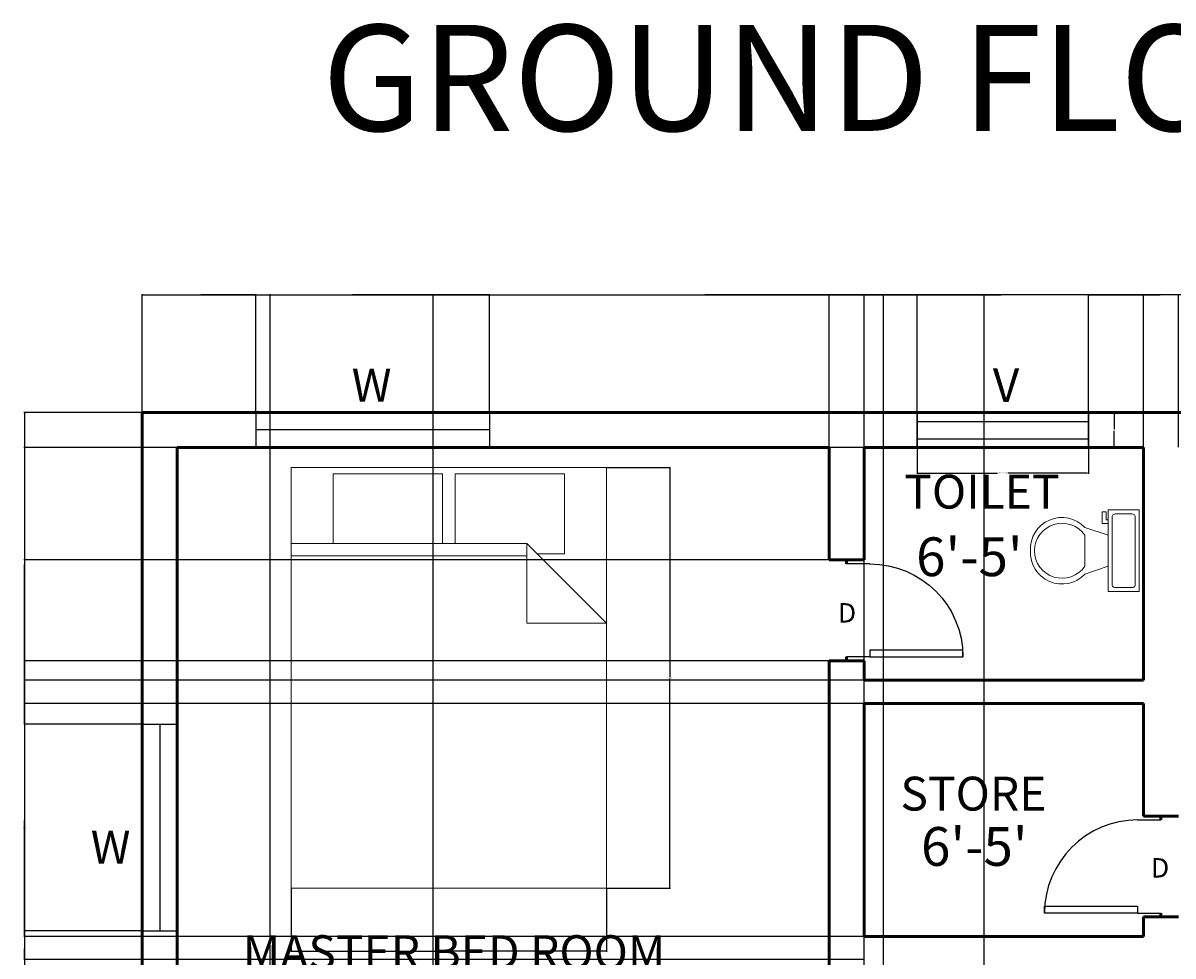
# Model space of a CAD drawing. Units: inches. Extents: x 2164 to 3752, y 2015 to 2629.
# Tile 3 of 8: x 2164 to 2461, y 2389 to 2629. Entities that reach past the tile are written whole.
import ezdxf
from ezdxf.enums import TextEntityAlignment as Align

# ---------------------------------------------------------------- set-up
doc = ezdxf.new("R2010")
doc.units = ezdxf.units.IN
for name, color, linetype, lineweight in [('A-ANNO-DIMS', 2, 'Continuous', 18), ('A-ANNO-TEXT', 7, 'Continuous', 25), ('A-AREA-IDEN', 3, 'Continuous', 25), ('A-DOOR', 3, 'Continuous', 25), ('A-FLOR-FIXT', 8, 'Continuous', 18), ('A-FURN', 8, 'Continuous', 18), ('A-GLAZ', 4, 'Continuous', 25), ('A-WALL', 7, 'Continuous', 50)]:
    doc.layers.add(name, color=color, linetype=linetype, lineweight=lineweight)
doc.styles.get("Standard").update_dxf_attribs({"font": 'arial.ttf'})
doc.dimstyles.get("Standard").update_dxf_attribs({"dimtxt": 0.18, "dimasz": 0.18, "dimexe": 0.18, "dimexo": 0.0625, "dimgap": 0.09, "dimtad": 0, "dimtih": 1, "dimtoh": 1, "dimdec": 4, "dimzin": 0, "dimdsep": 46, "dimtxsty": 'Standard', "dimcen": 0.09, "dimadec": 0, "dimazin": 0, "dimtfac": 1, "dimtdec": 4, "dimtofl": 0, "dimtmove": 0, "dimatfit": 3, "dimfxl": 1, "dimtolj": 1, "dimtzin": 0, "dimarcsym": 0})

# ---------------------------------------------------------------- blocks, each defined once
blk = doc.blocks.new('*U4')
for p, q in [((9.5, -6), (9.5, -2)), ((-10, -8.5), (-8, -8.5)), ((-10, -9.5), (-10, -8.5)), ((-8, -8.5), (-8, -8)), ((-7, -8), (-7, -9.5)), ((-4, -8), (-6, -14)), ((4, -8), (6, -14)), ((-7, -9.5), (-10, -9.5)), ((4, -14), (-4, -14))]:
    blk.add_line(p, q)
blk.add_lwpolyline([(10.5, -8), (10.5, 0), (-10.5, 0), (-10.5, -8)], close=True)
for points in [[(-9.5, -2), (-9.5, -6)], [(8.5, -1), (-8.5, -1)], [(-8.5, -7), (8.5, -7)]]:
    blk.add_lwpolyline(points)
for centre, radius, start, end in [((-8.625, -1.875), 0.8839, 81.8699, 188.1301), ((8.625, -1.875), 0.8839, 351.8699, 98.1301), ((-8.625, -6.125), 0.8839, 171.869898, 278.1301), ((8.625, -6.125), 0.8839, 261.8699, 8.1301), ((-0.4772, -19.9188), 8.0953, 133.01722, 273.38), ((0.0374, -19.8731), 7.127, 124.50543, 269.7), ((-0.0373, -19.8731), 7.127, 270.3, 55.4946), ((0.4773, -19.9188), 8.0953, 266.62, 46.9828)]:
    blk.add_arc(centre, radius, start, end)
blk = doc.blocks.new('*U2')
for p, q in [((0, 0), (0, -6)), ((24, 0), (24, -6))]:
    blk.add_line(p, q)
blk.add_lwpolyline([(0, 0), (0, 24), (1.75, 24), (1.75, 0)], close=True)
blk.add_arc((0, 0), 24, 0, 90)
blk = doc.blocks.new('Bed - Queen')
for p, q in [((0, -80.00003), (0, 0)), ((0, 0), (59.99999, 0)), ((59.99999, 0), (59.99999, -80.00003)), ((7.99999, -1.2), (28.79998, -1.2)), ((7.99999, -14.4), (7.99999, -1.2)), ((28.79998, -1.2), (28.79998, -14.4)), ((31.19999, -1.2), (51.99999, -1.2)), ((31.19999, -14.4), (31.19999, -1.2)), ((51.99999, -1.2), (51.99999, -16.4)), ((0, -14.4), (44.8, -14.4)), ((59.99999, -29.6), (44.8, -14.4)), ((44.8, -14.4), (44.8, -29.6)), ((44.8, -16.8), (0, -16.8)), ((51.99999, -16.4), (46.79936, -16.4)), ((44.8, -29.6), (59.99999, -29.6)), ((59.99999, -80.00003), (0, -80.00003))]:
    blk.add_line(p, q)
blk = doc.blocks.new('VENTILATOR')
for p, q in [((2394.78, 2528.72), (2394.78, 2519.72)), ((2438.92, 2528.72), (2438.92, 2519.72)), ((2394.78, 2526.43), (2438.92, 2526.43)), ((2438.92, 2521.87), (2394.78, 2521.87))]:
    blk.add_line(p, q)
blk = doc.blocks.new('*D23')
at = {"layer": 'A-ANNO-DIMS', "color": 0, "lineweight": -2, "transparency": 16777216}
for p, q in [((2314.85, 2514.51), (2331.22, 2514.51)), ((2331.04, 2514.33), (2331.04, 2460.51)), ((2331.04, 2406.31), (2331.04, 2460.13)), ((2314.85, 2406.13), (2331.22, 2406.13))]:
    blk.add_line(p, q, dxfattribs=at)
at = {"layer": 'A-ANNO-DIMS', "color": 0, "transparency": 16777216}
for points in [[(2331.01, 2514.33), (2331.07, 2514.33), (2331.04, 2514.51)], [(2331.01, 2406.31), (2331.07, 2406.31), (2331.04, 2406.13)]]:
    blk.add_solid(points, dxfattribs=at)
at = {"layer": 'Defpoints', "color": 0, "transparency": 16777216}
for p in [(2314.78, 2514.51), (2331.04, 2514.51), (2314.78, 2406.13)]:
    blk.add_point(p, dxfattribs=at)
at = {"layer": 'A-ANNO-DIMS', "color": 0, "transparency": 16777216, "insert": (2331.04, 2460.32), "char_height": 0.18, "attachment_point": 5}
blk.add_mtext('\\A1;QUEEN BED 108 TYP.', dxfattribs=at)
blk = doc.blocks.new('*D24')
at = {"layer": 'A-ANNO-DIMS', "color": 0, "lineweight": -2, "transparency": 16777216}
for p, q in [((2233.5, 2406.07), (2233.5, 2389.7)), ((2314.78, 2406.07), (2314.78, 2389.7)), ((2233.68, 2389.88), (2273.61, 2389.88)), ((2314.6, 2389.88), (2274.67, 2389.88))]:
    blk.add_line(p, q, dxfattribs=at)
at = {"layer": 'A-ANNO-DIMS', "color": 0, "transparency": 16777216}
for points in [[(2233.68, 2389.91), (2233.68, 2389.85), (2233.5, 2389.88)], [(2314.6, 2389.91), (2314.6, 2389.85), (2314.78, 2389.88)]]:
    blk.add_solid(points, dxfattribs=at)
at = {"layer": 'Defpoints', "color": 0, "transparency": 16777216}
for p in [(2233.5, 2406.13), (2314.78, 2406.13), (2314.78, 2389.88)]:
    blk.add_point(p, dxfattribs=at)
at = {"layer": 'A-ANNO-DIMS', "color": 0, "transparency": 16777216, "insert": (2274.14, 2389.88), "char_height": 0.18, "attachment_point": 5}
blk.add_mtext('\\A1;81 TYP.', dxfattribs=at)
blk = doc.blocks.new('*D35')
at = {"layer": 'A-ANNO-DIMS', "color": 0, "lineweight": -2, "transparency": 16777216}
for p, q in [((2394.78, 2519.65), (2394.78, 2512.92)), ((2438.92, 2519.65), (2438.92, 2512.92)), ((2394.96, 2513.1), (2415.49, 2513.1)), ((2438.74, 2513.1), (2418.21, 2513.1))]:
    blk.add_line(p, q, dxfattribs=at)
at = {"layer": 'A-ANNO-DIMS', "color": 0, "transparency": 16777216}
for points in [[(2394.96, 2513.13), (2394.96, 2513.07), (2394.78, 2513.1)], [(2438.74, 2513.13), (2438.74, 2513.07), (2438.92, 2513.1)]]:
    blk.add_solid(points, dxfattribs=at)
at = {"layer": 'Defpoints', "color": 0, "transparency": 16777216}
for p in [(2394.78, 2519.72), (2438.92, 2519.72), (2438.92, 2513.1)]:
    blk.add_point(p, dxfattribs=at)
at = {"layer": 'A-ANNO-DIMS', "color": 0, "transparency": 16777216, "insert": (2416.85, 2513.1), "char_height": 0.18, "attachment_point": 5}
blk.add_mtext('\\A1;VENTILATOR 44 TYP.', dxfattribs=at)
blk = doc.blocks.new('*D36')
at = {"layer": 'A-ANNO-DIMS', "color": 0, "lineweight": -2, "transparency": 16777216}
for p, q in [((2438.98, 2528.72), (2445.72, 2528.72)), ((2445.54, 2528.54), (2445.54, 2524.4)), ((2445.54, 2519.9), (2445.54, 2524.04)), ((2438.98, 2519.72), (2445.72, 2519.72))]:
    blk.add_line(p, q, dxfattribs=at)
at = {"layer": 'A-ANNO-DIMS', "color": 0, "transparency": 16777216}
for points in [[(2445.51, 2528.54), (2445.57, 2528.54), (2445.54, 2528.72)], [(2445.51, 2519.9), (2445.57, 2519.9), (2445.54, 2519.72)]]:
    blk.add_solid(points, dxfattribs=at)
at = {"layer": 'Defpoints', "color": 0, "transparency": 16777216}
for p in [(2438.92, 2528.72), (2445.54, 2528.72), (2438.92, 2519.72)]:
    blk.add_point(p, dxfattribs=at)
at = {"layer": 'A-ANNO-DIMS', "color": 0, "transparency": 16777216, "insert": (2445.54, 2524.22), "char_height": 0.18, "attachment_point": 5}
blk.add_mtext('\\A1;9 TYP.', dxfattribs=at)
blk = doc.blocks.new('*D47')
at = {"layer": 'A-ANNO-DIMS', "color": 0, "lineweight": -2, "transparency": 16777216}
for p, q in [((2195.11, 2528.78), (2195.11, 2559.25)), ((2195.29, 2559.07), (2209.27, 2559.07)), ((2224.19, 2559.07), (2210.2, 2559.07)), ((2224.37, 2528.78), (2224.37, 2559.25))]:
    blk.add_line(p, q, dxfattribs=at)
at = {"layer": 'A-ANNO-DIMS', "color": 0, "transparency": 16777216}
for points in [[(2195.29, 2559.1), (2195.29, 2559.04), (2195.11, 2559.07)], [(2224.19, 2559.1), (2224.19, 2559.04), (2224.37, 2559.07)]]:
    blk.add_solid(points, dxfattribs=at)
at = {"layer": 'Defpoints', "color": 0, "transparency": 16777216}
for p in [(2224.37, 2559.07), (2195.11, 2528.72), (2224.37, 2528.72)]:
    blk.add_point(p, dxfattribs=at)
at = {"layer": 'A-ANNO-DIMS', "color": 0, "transparency": 16777216, "insert": (2209.74, 2559.07), "char_height": 0.18, "attachment_point": 5}
blk.add_mtext('\\A1;29.254', dxfattribs=at)
blk = doc.blocks.new('*D48')
at = {"layer": 'A-ANNO-DIMS', "color": 0, "lineweight": -2, "transparency": 16777216}
for p, q in [((2224.37, 2528.78), (2224.37, 2559.25)), ((2224.55, 2559.07), (2254.08, 2559.07)), ((2284.4, 2559.07), (2254.87, 2559.07)), ((2284.58, 2528.78), (2284.58, 2559.25))]:
    blk.add_line(p, q, dxfattribs=at)
at = {"layer": 'A-ANNO-DIMS', "color": 0, "transparency": 16777216}
for points in [[(2224.55, 2559.1), (2224.55, 2559.04), (2224.37, 2559.07)], [(2284.4, 2559.1), (2284.4, 2559.04), (2284.58, 2559.07)]]:
    blk.add_solid(points, dxfattribs=at)
at = {"layer": 'Defpoints', "color": 0, "transparency": 16777216}
for p in [(2284.58, 2559.07), (2224.37, 2528.72), (2284.58, 2528.72)]:
    blk.add_point(p, dxfattribs=at)
at = {"layer": 'A-ANNO-DIMS', "color": 0, "transparency": 16777216, "insert": (2254.47, 2559.07), "char_height": 0.18, "attachment_point": 5}
blk.add_mtext('\\A1;60.22', dxfattribs=at)
blk = doc.blocks.new('*D49')
at = {"layer": 'A-ANNO-DIMS', "color": 0, "lineweight": -2, "transparency": 16777216}
for p, q in [((2284.58, 2528.78), (2284.58, 2559.25)), ((2284.76, 2559.07), (2339.3, 2559.07)), ((2394.6, 2559.07), (2340.07, 2559.07)), ((2394.78, 2528.78), (2394.78, 2559.25))]:
    blk.add_line(p, q, dxfattribs=at)
at = {"layer": 'A-ANNO-DIMS', "color": 0, "transparency": 16777216}
for points in [[(2284.76, 2559.1), (2284.76, 2559.04), (2284.58, 2559.07)], [(2394.6, 2559.1), (2394.6, 2559.04), (2394.78, 2559.07)]]:
    blk.add_solid(points, dxfattribs=at)
at = {"layer": 'Defpoints', "color": 0, "transparency": 16777216}
for p in [(2394.78, 2559.07), (2284.58, 2528.72), (2394.78, 2528.72)]:
    blk.add_point(p, dxfattribs=at)
at = {"layer": 'A-ANNO-DIMS', "color": 0, "transparency": 16777216, "insert": (2339.68, 2559.07), "char_height": 0.18, "attachment_point": 5}
blk.add_mtext('\\A1;110.2', dxfattribs=at)
blk = doc.blocks.new('*D50')
at = {"layer": 'A-ANNO-DIMS', "color": 0, "lineweight": -2, "transparency": 16777216}
for p, q in [((2394.78, 2528.78), (2394.78, 2559.25)), ((2394.96, 2559.07), (2416.45, 2559.07)), ((2438.74, 2559.07), (2417.25, 2559.07)), ((2438.92, 2528.78), (2438.92, 2559.25))]:
    blk.add_line(p, q, dxfattribs=at)
at = {"layer": 'A-ANNO-DIMS', "color": 0, "transparency": 16777216}
for points in [[(2394.96, 2559.1), (2394.96, 2559.04), (2394.78, 2559.07)], [(2438.74, 2559.1), (2438.74, 2559.04), (2438.92, 2559.07)]]:
    blk.add_solid(points, dxfattribs=at)
at = {"layer": 'Defpoints', "color": 0, "transparency": 16777216}
for p in [(2438.92, 2559.07), (2394.78, 2528.72), (2438.92, 2528.72)]:
    blk.add_point(p, dxfattribs=at)
at = {"layer": 'A-ANNO-DIMS', "color": 0, "transparency": 16777216, "insert": (2416.85, 2559.07), "char_height": 0.18, "attachment_point": 5}
blk.add_mtext('\\A1;44.13', dxfattribs=at)
blk = doc.blocks.new('*D51')
at = {"layer": 'A-ANNO-DIMS', "color": 0, "lineweight": -2, "transparency": 16777216}
for p, q in [((2438.92, 2528.78), (2438.92, 2559.25)), ((2439.1, 2559.07), (2453.99, 2559.07)), ((2469.68, 2559.07), (2454.78, 2559.07)), ((2469.86, 2528.78), (2469.86, 2559.25))]:
    blk.add_line(p, q, dxfattribs=at)
at = {"layer": 'A-ANNO-DIMS', "color": 0, "transparency": 16777216}
for points in [[(2439.1, 2559.1), (2439.1, 2559.04), (2438.92, 2559.07)], [(2469.68, 2559.1), (2469.68, 2559.04), (2469.86, 2559.07)]]:
    blk.add_solid(points, dxfattribs=at)
at = {"layer": 'Defpoints', "color": 0, "transparency": 16777216}
for p in [(2469.86, 2559.07), (2438.92, 2528.72), (2469.86, 2528.72)]:
    blk.add_point(p, dxfattribs=at)
at = {"layer": 'A-ANNO-DIMS', "color": 0, "transparency": 16777216, "insert": (2454.39, 2559.07), "char_height": 0.18, "attachment_point": 5}
blk.add_mtext('\\A1;30.94', dxfattribs=at)
blk = doc.blocks.new('*D54')
at = {"layer": 'A-ANNO-DIMS', "color": 0, "lineweight": -2, "transparency": 16777216}
for p, q in [((2195.11, 2528.78), (2195.11, 2559.25)), ((2195.29, 2559.07), (2392.82, 2559.07)), ((2590.93, 2559.07), (2393.4, 2559.07)), ((2591.11, 2528.78), (2591.11, 2559.25))]:
    blk.add_line(p, q, dxfattribs=at)
at = {"layer": 'A-ANNO-DIMS', "color": 0, "transparency": 16777216}
for points in [[(2195.29, 2559.1), (2195.29, 2559.04), (2195.11, 2559.07)], [(2590.93, 2559.1), (2590.93, 2559.04), (2591.11, 2559.07)]]:
    blk.add_solid(points, dxfattribs=at)
at = {"layer": 'Defpoints', "color": 0, "transparency": 16777216}
for p in [(2591.11, 2559.07), (2195.11, 2528.72), (2591.11, 2528.72)]:
    blk.add_point(p, dxfattribs=at)
at = {"layer": 'A-ANNO-DIMS', "color": 0, "transparency": 16777216, "insert": (2393.11, 2559.07), "char_height": 0.18, "attachment_point": 5}
blk.add_mtext('\\A1;396', dxfattribs=at)
blk = doc.blocks.new('*D55')
at = {"layer": 'A-ANNO-DIMS', "color": 0, "lineweight": -2, "transparency": 16777216}
for p, q in [((2372.11, 2519.78), (2372.11, 2559.25)), ((2372.29, 2559.07), (2376.46, 2559.07)), ((2380.93, 2559.07), (2376.76, 2559.07)), ((2381.11, 2519.78), (2381.11, 2559.25))]:
    blk.add_line(p, q, dxfattribs=at)
at = {"layer": 'A-ANNO-DIMS', "color": 0, "transparency": 16777216}
for points in [[(2372.29, 2559.1), (2372.29, 2559.04), (2372.11, 2559.07)], [(2380.93, 2559.1), (2380.93, 2559.04), (2381.11, 2559.07)]]:
    blk.add_solid(points, dxfattribs=at)
at = {"layer": 'Defpoints', "color": 0, "transparency": 16777216}
for p in [(2381.11, 2559.07), (2372.11, 2519.72), (2381.11, 2519.72)]:
    blk.add_point(p, dxfattribs=at)
at = {"layer": 'A-ANNO-DIMS', "color": 0, "transparency": 16777216, "insert": (2376.61, 2559.07), "char_height": 0.18, "attachment_point": 5}
blk.add_mtext('\\A1;9', dxfattribs=at)
blk = doc.blocks.new('*D56')
at = {"layer": 'A-ANNO-DIMS', "color": 0, "lineweight": -2, "transparency": 16777216}
for p, q in [((2381.11, 2519.78), (2381.11, 2559.25)), ((2381.29, 2559.07), (2387.56, 2559.07)), ((2394.6, 2559.07), (2388.33, 2559.07)), ((2394.78, 2519.78), (2394.78, 2559.25))]:
    blk.add_line(p, q, dxfattribs=at)
at = {"layer": 'A-ANNO-DIMS', "color": 0, "transparency": 16777216}
for points in [[(2381.29, 2559.1), (2381.29, 2559.04), (2381.11, 2559.07)], [(2394.6, 2559.1), (2394.6, 2559.04), (2394.78, 2559.07)]]:
    blk.add_solid(points, dxfattribs=at)
at = {"layer": 'Defpoints', "color": 0, "transparency": 16777216}
for p in [(2394.78, 2559.07), (2381.11, 2519.72), (2394.78, 2519.72)]:
    blk.add_point(p, dxfattribs=at)
at = {"layer": 'A-ANNO-DIMS', "color": 0, "transparency": 16777216, "insert": (2387.95, 2559.07), "char_height": 0.18, "attachment_point": 5}
blk.add_mtext('\\A1;13.67', dxfattribs=at)
blk = doc.blocks.new('*D57')
at = {"layer": 'A-ANNO-DIMS', "color": 0, "lineweight": -2, "transparency": 16777216}
for p, q in [((2438.92, 2519.78), (2438.92, 2559.25)), ((2439.1, 2559.07), (2445.56, 2559.07)), ((2452.93, 2559.07), (2446.47, 2559.07)), ((2453.11, 2519.78), (2453.11, 2559.25))]:
    blk.add_line(p, q, dxfattribs=at)
at = {"layer": 'A-ANNO-DIMS', "color": 0, "transparency": 16777216}
for points in [[(2439.1, 2559.1), (2439.1, 2559.04), (2438.92, 2559.07)], [(2452.93, 2559.1), (2452.93, 2559.04), (2453.11, 2559.07)]]:
    blk.add_solid(points, dxfattribs=at)
at = {"layer": 'Defpoints', "color": 0, "transparency": 16777216}
for p in [(2453.11, 2559.07), (2438.92, 2519.72), (2453.11, 2519.72)]:
    blk.add_point(p, dxfattribs=at)
at = {"layer": 'A-ANNO-DIMS', "color": 0, "transparency": 16777216, "insert": (2446.01, 2559.07), "char_height": 0.18, "attachment_point": 5}
blk.add_mtext('\\A1;14.196', dxfattribs=at)
blk = doc.blocks.new('*D58')
at = {"layer": 'A-ANNO-DIMS', "color": 0, "lineweight": -2, "transparency": 16777216}
for p, q in [((2453.11, 2519.78), (2453.11, 2559.25)), ((2453.29, 2559.07), (2457.46, 2559.07)), ((2461.93, 2559.07), (2457.76, 2559.07)), ((2462.11, 2519.78), (2462.11, 2559.25))]:
    blk.add_line(p, q, dxfattribs=at)
at = {"layer": 'A-ANNO-DIMS', "color": 0, "transparency": 16777216}
for points in [[(2453.29, 2559.1), (2453.29, 2559.04), (2453.11, 2559.07)], [(2461.93, 2559.1), (2461.93, 2559.04), (2462.11, 2559.07)]]:
    blk.add_solid(points, dxfattribs=at)
at = {"layer": 'Defpoints', "color": 0, "transparency": 16777216}
for p in [(2462.11, 2559.07), (2453.11, 2519.72), (2462.11, 2519.72)]:
    blk.add_point(p, dxfattribs=at)
at = {"layer": 'A-ANNO-DIMS', "color": 0, "transparency": 16777216, "insert": (2457.61, 2559.07), "char_height": 0.18, "attachment_point": 5}
blk.add_mtext('\\A1;9', dxfattribs=at)
blk = doc.blocks.new('*D72')
at = {"layer": 'A-ANNO-DIMS', "color": 0, "lineweight": -2, "transparency": 16777216}
for p, q in [((2195.05, 2395.15), (2164.58, 2395.15)), ((2164.76, 2394.97), (2164.76, 2337.1)), ((2164.76, 2278.87), (2164.76, 2336.74)), ((2195.05, 2278.69), (2164.58, 2278.69))]:
    blk.add_line(p, q, dxfattribs=at)
at = {"layer": 'A-ANNO-DIMS', "color": 0, "transparency": 16777216}
for points in [[(2164.73, 2394.97), (2164.79, 2394.97), (2164.76, 2395.15)], [(2164.73, 2278.87), (2164.79, 2278.87), (2164.76, 2278.69)]]:
    blk.add_solid(points, dxfattribs=at)
at = {"layer": 'Defpoints', "color": 0, "transparency": 16777216}
for p in [(2164.76, 2395.15), (2195.11, 2395.15), (2195.11, 2278.69)]:
    blk.add_point(p, dxfattribs=at)
at = {"layer": 'A-ANNO-DIMS', "color": 0, "transparency": 16777216, "insert": (2164.76, 2336.92), "char_height": 0.18, "attachment_point": 5}
blk.add_mtext('\\A1;116.47', dxfattribs=at)
blk = doc.blocks.new('*D73')
at = {"layer": 'A-ANNO-DIMS', "color": 0, "lineweight": -2, "transparency": 16777216}
for p, q in [((2195.05, 2448.4), (2164.58, 2448.4)), ((2164.76, 2448.22), (2164.76, 2421.96)), ((2164.76, 2395.33), (2164.76, 2421.59)), ((2195.05, 2395.15), (2164.58, 2395.15))]:
    blk.add_line(p, q, dxfattribs=at)
at = {"layer": 'A-ANNO-DIMS', "color": 0, "transparency": 16777216}
for points in [[(2164.73, 2448.22), (2164.79, 2448.22), (2164.76, 2448.4)], [(2164.73, 2395.33), (2164.79, 2395.33), (2164.76, 2395.15)]]:
    blk.add_solid(points, dxfattribs=at)
at = {"layer": 'Defpoints', "color": 0, "transparency": 16777216}
for p in [(2164.76, 2448.4), (2195.11, 2448.4), (2195.11, 2395.15)]:
    blk.add_point(p, dxfattribs=at)
at = {"layer": 'A-ANNO-DIMS', "color": 0, "transparency": 16777216, "insert": (2164.76, 2421.78), "char_height": 0.18, "attachment_point": 5}
blk.add_mtext('\\A1;53.25', dxfattribs=at)
blk = doc.blocks.new('*D74')
at = {"layer": 'A-ANNO-DIMS', "color": 0, "lineweight": -2, "transparency": 16777216}
for p, q in [((2195.05, 2528.72), (2164.58, 2528.72)), ((2164.76, 2528.54), (2164.76, 2488.74)), ((2164.76, 2448.58), (2164.76, 2488.38)), ((2195.05, 2448.4), (2164.58, 2448.4))]:
    blk.add_line(p, q, dxfattribs=at)
at = {"layer": 'A-ANNO-DIMS', "color": 0, "transparency": 16777216}
for points in [[(2164.73, 2528.54), (2164.79, 2528.54), (2164.76, 2528.72)], [(2164.73, 2448.58), (2164.79, 2448.58), (2164.76, 2448.4)]]:
    blk.add_solid(points, dxfattribs=at)
at = {"layer": 'Defpoints', "color": 0, "transparency": 16777216}
for p in [(2164.76, 2528.72), (2195.11, 2528.72), (2195.11, 2448.4)]:
    blk.add_point(p, dxfattribs=at)
at = {"layer": 'A-ANNO-DIMS', "color": 0, "transparency": 16777216, "insert": (2164.76, 2488.56), "char_height": 0.18, "attachment_point": 5}
blk.add_mtext('\\A1;80.32', dxfattribs=at)
blk = doc.blocks.new('*D75')
at = {"layer": 'A-ANNO-DIMS', "color": 0, "lineweight": -2, "transparency": 16777216}
for p, q in [((2195.05, 2528.72), (2164.58, 2528.72)), ((2164.76, 2528.54), (2164.76, 2287.4)), ((2164.76, 2045.9), (2164.76, 2287.04)), ((2195.05, 2045.72), (2164.58, 2045.72))]:
    blk.add_line(p, q, dxfattribs=at)
at = {"layer": 'A-ANNO-DIMS', "color": 0, "transparency": 16777216}
for points in [[(2164.73, 2528.54), (2164.79, 2528.54), (2164.76, 2528.72)], [(2164.73, 2045.9), (2164.79, 2045.9), (2164.76, 2045.72)]]:
    blk.add_solid(points, dxfattribs=at)
at = {"layer": 'Defpoints', "color": 0, "transparency": 16777216}
for p in [(2164.76, 2528.72), (2195.11, 2528.72), (2195.11, 2045.72)]:
    blk.add_point(p, dxfattribs=at)
at = {"layer": 'A-ANNO-DIMS', "color": 0, "transparency": 16777216, "insert": (2164.76, 2287.22), "char_height": 0.18, "attachment_point": 5}
blk.add_mtext('\\A1;483', dxfattribs=at)
blk = doc.blocks.new('*D88')
at = {"layer": 'A-ANNO-DIMS', "color": 0, "lineweight": -2, "transparency": 16777216}
for p, q in [((2381.05, 2393.72), (2164.58, 2393.72)), ((2164.76, 2393.54), (2164.76, 2390.9)), ((2164.76, 2387.9), (2164.76, 2390.54)), ((2381.05, 2387.72), (2164.58, 2387.72))]:
    blk.add_line(p, q, dxfattribs=at)
at = {"layer": 'A-ANNO-DIMS', "color": 0, "transparency": 16777216}
for points in [[(2164.73, 2393.54), (2164.79, 2393.54), (2164.76, 2393.72)], [(2164.73, 2387.9), (2164.79, 2387.9), (2164.76, 2387.72)]]:
    blk.add_solid(points, dxfattribs=at)
at = {"layer": 'Defpoints', "color": 0, "transparency": 16777216}
for p in [(2164.76, 2393.72), (2381.11, 2393.72), (2381.11, 2387.72)]:
    blk.add_point(p, dxfattribs=at)
at = {"layer": 'A-ANNO-DIMS', "color": 0, "transparency": 16777216, "insert": (2164.76, 2390.72), "char_height": 0.18, "attachment_point": 5}
blk.add_mtext('\\A1;6', dxfattribs=at)
blk = doc.blocks.new('*D89')
at = {"layer": 'A-ANNO-DIMS', "color": 0, "lineweight": -2, "transparency": 16777216}
for p, q in [((2381.05, 2453.72), (2164.58, 2453.72)), ((2164.76, 2453.54), (2164.76, 2423.9)), ((2164.76, 2393.9), (2164.76, 2423.54)), ((2381.05, 2393.72), (2164.58, 2393.72))]:
    blk.add_line(p, q, dxfattribs=at)
at = {"layer": 'A-ANNO-DIMS', "color": 0, "transparency": 16777216}
for points in [[(2164.73, 2453.54), (2164.79, 2453.54), (2164.76, 2453.72)], [(2164.73, 2393.9), (2164.79, 2393.9), (2164.76, 2393.72)]]:
    blk.add_solid(points, dxfattribs=at)
at = {"layer": 'Defpoints', "color": 0, "transparency": 16777216}
for p in [(2164.76, 2453.72), (2381.11, 2453.72), (2381.11, 2393.72)]:
    blk.add_point(p, dxfattribs=at)
at = {"layer": 'A-ANNO-DIMS', "color": 0, "transparency": 16777216, "insert": (2164.76, 2423.72), "char_height": 0.18, "attachment_point": 5}
blk.add_mtext('\\A1;60', dxfattribs=at)
blk = doc.blocks.new('*D90')
at = {"layer": 'A-ANNO-DIMS', "color": 0, "lineweight": -2, "transparency": 16777216}
for p, q in [((2381.05, 2459.72), (2164.58, 2459.72)), ((2164.76, 2459.54), (2164.76, 2456.9)), ((2164.76, 2453.9), (2164.76, 2456.54)), ((2381.05, 2453.72), (2164.58, 2453.72))]:
    blk.add_line(p, q, dxfattribs=at)
at = {"layer": 'A-ANNO-DIMS', "color": 0, "transparency": 16777216}
for points in [[(2164.73, 2459.54), (2164.79, 2459.54), (2164.76, 2459.72)], [(2164.73, 2453.9), (2164.79, 2453.9), (2164.76, 2453.72)]]:
    blk.add_solid(points, dxfattribs=at)
at = {"layer": 'Defpoints', "color": 0, "transparency": 16777216}
for p in [(2164.76, 2459.72), (2381.11, 2459.72), (2381.11, 2453.72)]:
    blk.add_point(p, dxfattribs=at)
at = {"layer": 'A-ANNO-DIMS', "color": 0, "transparency": 16777216, "insert": (2164.76, 2456.72), "char_height": 0.18, "attachment_point": 5}
blk.add_mtext('\\A1;6', dxfattribs=at)
blk = doc.blocks.new('*D91')
at = {"layer": 'A-ANNO-DIMS', "color": 0, "lineweight": -2, "transparency": 16777216}
for p, q in [((2381.05, 2519.72), (2164.58, 2519.72)), ((2164.76, 2519.54), (2164.76, 2489.9)), ((2164.76, 2459.9), (2164.76, 2489.54)), ((2381.05, 2459.72), (2164.58, 2459.72))]:
    blk.add_line(p, q, dxfattribs=at)
at = {"layer": 'A-ANNO-DIMS', "color": 0, "transparency": 16777216}
for points in [[(2164.73, 2519.54), (2164.79, 2519.54), (2164.76, 2519.72)], [(2164.73, 2459.9), (2164.79, 2459.9), (2164.76, 2459.72)]]:
    blk.add_solid(points, dxfattribs=at)
at = {"layer": 'Defpoints', "color": 0, "transparency": 16777216}
for p in [(2164.76, 2519.72), (2381.11, 2519.72), (2381.11, 2459.72)]:
    blk.add_point(p, dxfattribs=at)
at = {"layer": 'A-ANNO-DIMS', "color": 0, "transparency": 16777216, "insert": (2164.76, 2489.72), "char_height": 0.18, "attachment_point": 5}
blk.add_mtext('\\A1;60', dxfattribs=at)
blk = doc.blocks.new('*D92')
at = {"layer": 'A-ANNO-DIMS', "color": 0, "lineweight": -2, "transparency": 16777216}
for p, q in [((2228.11, 2327.78), (2228.11, 2559.25)), ((2228.29, 2559.07), (2248.89, 2559.07)), ((2269.93, 2559.07), (2249.33, 2559.07)), ((2270.11, 2327.78), (2270.11, 2559.25))]:
    blk.add_line(p, q, dxfattribs=at)
at = {"layer": 'A-ANNO-DIMS', "color": 0, "transparency": 16777216}
for points in [[(2228.29, 2559.1), (2228.29, 2559.04), (2228.11, 2559.07)], [(2269.93, 2559.1), (2269.93, 2559.04), (2270.11, 2559.07)]]:
    blk.add_solid(points, dxfattribs=at)
at = {"layer": 'Defpoints', "color": 0, "transparency": 16777216}
for p in [(2270.11, 2559.07), (2228.11, 2327.72), (2270.11, 2327.72)]:
    blk.add_point(p, dxfattribs=at)
at = {"layer": 'A-ANNO-DIMS', "color": 0, "transparency": 16777216, "insert": (2249.11, 2559.07), "char_height": 0.18, "attachment_point": 5}
blk.add_mtext('\\A1;42', dxfattribs=at)
blk = doc.blocks.new('*D93')
at = {"layer": 'A-ANNO-DIMS', "color": 0, "lineweight": -2, "transparency": 16777216}
for p, q in [((2381.11, 2327.78), (2381.11, 2559.25)), ((2381.29, 2559.07), (2383.46, 2559.07)), ((2385.93, 2559.07), (2383.76, 2559.07)), ((2386.11, 2327.78), (2386.11, 2559.25))]:
    blk.add_line(p, q, dxfattribs=at)
at = {"layer": 'A-ANNO-DIMS', "color": 0, "transparency": 16777216}
for points in [[(2381.29, 2559.1), (2381.29, 2559.04), (2381.11, 2559.07)], [(2385.93, 2559.1), (2385.93, 2559.04), (2386.11, 2559.07)]]:
    blk.add_solid(points, dxfattribs=at)
at = {"layer": 'Defpoints', "color": 0, "transparency": 16777216}
for p in [(2386.11, 2559.07), (2381.11, 2327.72), (2386.11, 2327.72)]:
    blk.add_point(p, dxfattribs=at)
at = {"layer": 'A-ANNO-DIMS', "color": 0, "transparency": 16777216, "insert": (2383.61, 2559.07), "char_height": 0.18, "attachment_point": 5}
blk.add_mtext('\\A1;5', dxfattribs=at)
blk = doc.blocks.new('*D94')
at = {"layer": 'A-ANNO-DIMS', "color": 0, "lineweight": -2, "transparency": 16777216}
for p, q in [((2386.11, 2327.78), (2386.11, 2559.25)), ((2386.29, 2559.07), (2398.89, 2559.07)), ((2411.93, 2559.07), (2399.33, 2559.07)), ((2412.11, 2327.78), (2412.11, 2559.25))]:
    blk.add_line(p, q, dxfattribs=at)
at = {"layer": 'A-ANNO-DIMS', "color": 0, "transparency": 16777216}
for points in [[(2386.29, 2559.1), (2386.29, 2559.04), (2386.11, 2559.07)], [(2411.93, 2559.1), (2411.93, 2559.04), (2412.11, 2559.07)]]:
    blk.add_solid(points, dxfattribs=at)
at = {"layer": 'Defpoints', "color": 0, "transparency": 16777216}
for p in [(2412.11, 2559.07), (2386.11, 2327.72), (2412.11, 2327.72)]:
    blk.add_point(p, dxfattribs=at)
at = {"layer": 'A-ANNO-DIMS', "color": 0, "transparency": 16777216, "insert": (2399.11, 2559.07), "char_height": 0.18, "attachment_point": 5}
blk.add_mtext('\\A1;26', dxfattribs=at)
blk = doc.blocks.new('*D96')
at = {"layer": 'A-ANNO-DIMS', "color": 0, "lineweight": -2, "transparency": 16777216}
for p, q in [((2372.05, 2490.72), (2164.58, 2490.72)), ((2164.76, 2490.54), (2164.76, 2477.9)), ((2164.76, 2464.9), (2164.76, 2477.54)), ((2372.05, 2464.72), (2164.58, 2464.72))]:
    blk.add_line(p, q, dxfattribs=at)
at = {"layer": 'A-ANNO-DIMS', "color": 0, "transparency": 16777216}
for points in [[(2164.73, 2490.54), (2164.79, 2490.54), (2164.76, 2490.72)], [(2164.73, 2464.9), (2164.79, 2464.9), (2164.76, 2464.72)]]:
    blk.add_solid(points, dxfattribs=at)
at = {"layer": 'Defpoints', "color": 0, "transparency": 16777216}
for p in [(2164.76, 2490.72), (2372.11, 2490.72), (2372.11, 2464.72)]:
    blk.add_point(p, dxfattribs=at)
at = {"layer": 'A-ANNO-DIMS', "color": 0, "transparency": 16777216, "insert": (2164.76, 2477.72), "char_height": 0.18, "attachment_point": 5}
blk.add_mtext('\\A1;26', dxfattribs=at)

msp = doc.modelspace()

# ---------------------------------------------------------------- linework, layer by layer
at = {"layer": 'A-GLAZ'}
for p, q in [((2224.3652, 2528.7172), (2224.3652, 2519.7172)), ((2284.5822, 2528.7172), (2284.5822, 2519.7172)), ((2284.5822, 2524.2172), (2224.3652, 2524.2172)), ((2195.1113, 2448.3998), (2204.1113, 2448.3998)), ((2199.6113, 2448.3998), (2199.6113, 2395.1516)), ((2195.1113, 2395.1516), (2204.1113, 2395.1516))]:
    msp.add_line(p, q, dxfattribs=at)
at = {"layer": 'A-WALL'}
for p, q in [((2195.1113, 2528.7172), (2591.1113, 2528.7172)), ((2195.1113, 2528.7172), (2195.1113, 2045.7172)), ((2204.1113, 2519.7172), (2372.1113, 2519.7172)), ((2204.1113, 2519.7172), (2204.1113, 2327.7172)), ((2372.1113, 2519.7172), (2372.1113, 2490.7172)), ((2381.1113, 2519.7172), (2453.1113, 2519.7172)), ((2381.1113, 2519.7172), (2381.1113, 2490.7172)), ((2453.1113, 2519.7172), (2453.1113, 2459.7172)), ((2372.1113, 2490.7172), (2381.1113, 2490.7172)), ((2376.6113, 2489.7172), (2376.6113, 2490.7172)), ((2376.6113, 2464.7172), (2376.6113, 2465.7172)), ((2372.1113, 2464.7172), (2372.1113, 2327.7172)), ((2381.1113, 2464.7172), (2372.1113, 2464.7172)), ((2381.1113, 2464.7172), (2381.1113, 2459.7172)), ((2381.1113, 2459.7172), (2453.1113, 2459.7172)), ((2381.1113, 2453.7172), (2453.1113, 2453.7172)), ((2381.1113, 2453.7172), (2381.1113, 2393.7172)), ((2453.1113, 2453.7172), (2453.1113, 2424.7172)), ((2453.1113, 2424.7172), (2462.1113, 2424.7172)), ((2457.6113, 2423.7172), (2457.6113, 2424.7172)), ((2453.1113, 2398.7172), (2453.1113, 2393.7172)), ((2453.1113, 2398.7172), (2462.1113, 2398.7172)), ((2457.6113, 2398.7172), (2457.6113, 2399.7172)), ((2381.1113, 2393.7172), (2453.1113, 2393.7172))]:
    msp.add_line(p, q, dxfattribs=at)

# ---------------------------------------------------------------- block references
at = {"layer": 'A-DOOR', "xscale": -1, "rotation": 270}
msp.add_blockref('*U2', (2382.6113, 2465.7172), dxfattribs=at)
at = {"layer": 'A-DOOR', "rotation": 90.00000000000003}
msp.add_blockref('*U2', (2451.6113, 2399.7172), dxfattribs=at)
at = {"layer": 'A-FLOR-FIXT', "rotation": 270}
msp.add_blockref('*U4', (2452.0184, 2493.0967), dxfattribs=at)
at = {"layer": 'A-FURN', "xscale": 1.354750275868299, "yscale": 1.354750275868299, "zscale": 1.354750275868299}
msp.add_blockref('Bed - Queen', (2233.4983, 2514.5121), dxfattribs=at)
at = {"layer": 'A-GLAZ'}
msp.add_blockref('VENTILATOR', (0, 0), dxfattribs=at)

# ---------------------------------------------------------------- texts
at = {"layer": 'A-ANNO-TEXT'}
for s, height, p in [('GROUND FLOOR', 27.32215, (2383.759, 2611.4091)), ('W', 8.5558, (2254.2164, 2534.6404)), ('V', 8.7141, (2417.7002, 2534.6538)), ('W', 8.5558, (2186.9603, 2415.5987))]:
    msp.add_text(s, height=height, dxfattribs=at).set_placement(p, align=Align.MIDDLE)
for p in [(2374.3839, 2474.5937), (2455.0587, 2408.8828)]:
    msp.add_text('D', height=5, dxfattribs=at).set_placement(p)
at = {"layer": 'A-AREA-IDEN'}
for s, height, p in [('TOILET', 8.72285, (2391.4791, 2503.9584)), ("6'-5'", 10, (2394.5279, 2486.5498)), ('STORE', 8.72285, (2390.4915, 2426.144)), ("6'-5'", 10, (2395.7998, 2411.8926)), ('MASTER BED ROOM', 8.722848, (2221.017, 2385.2901))]:
    msp.add_text(s, height=height, dxfattribs=at).set_placement(p)

# ---------------------------------------------------------------- dimensions: what is measured, and where the dimension line sits
at = {"layer": 'A-ANNO-DIMS'}
for base, p1, p2, override, picture, middle in [((2224.3652, 2559.0672), (2195.1113, 2528.7172), (2224.3652, 2528.7172), {"dimdec": 3, "dimlfac": 1, "dimrnd": 0, "dimzin": 0, "dimdsep": 46, "dimlunit": 2}, '*D47', (2209.7382, 2559.0672)), ((2591.1113, 2559.0672), (2195.1113, 2528.7172), (2591.1113, 2528.7172), {"dimdec": 0, "dimlfac": 1, "dimrnd": 0, "dimzin": 0, "dimdsep": 46, "dimlunit": 2}, '*D54', (2393.1113, 2559.0672)), ((2284.5822, 2559.0672), (2224.3652, 2528.7172), (2284.5822, 2528.7172), {"dimdec": 2, "dimlfac": 1, "dimrnd": 0, "dimzin": 0, "dimdsep": 46, "dimlunit": 2}, '*D48', (2254.4737, 2559.0672)), ((2270.1108, 2559.0672), (2228.1113, 2327.7172), (2270.1108, 2327.7172), {"dimdec": 0, "dimlfac": 1, "dimrnd": 0, "dimzin": 0, "dimdsep": 46, "dimlunit": 2}, '*D92', (2249.1111, 2559.0672)), ((2394.782, 2559.0672), (2284.5822, 2528.7172), (2394.782, 2528.7172), {"dimdec": 1, "dimlfac": 1, "dimrnd": 0, "dimzin": 0, "dimdsep": 46, "dimlunit": 2}, '*D49', (2339.6821, 2559.0672)), ((2381.1113, 2559.0672), (2372.1113, 2519.7172), (2381.1113, 2519.7172), {"dimdec": 0, "dimlfac": 1, "dimrnd": 0, "dimzin": 0, "dimdsep": 46, "dimlunit": 2}, '*D55', (2376.6113, 2559.0672)), ((2394.782, 2559.0672), (2381.1113, 2519.7172), (2394.782, 2519.7172), {"dimdec": 2, "dimlfac": 1, "dimrnd": 0, "dimzin": 0, "dimdsep": 46, "dimlunit": 2}, '*D56', (2387.9467, 2559.0672)), ((2386.1113, 2559.0672), (2381.1113, 2327.7172), (2386.1113, 2327.7172), {"dimdec": 0, "dimlfac": 1, "dimrnd": 0, "dimzin": 0, "dimdsep": 46, "dimlunit": 2}, '*D93', (2383.6113, 2559.0672)), ((2412.1112, 2559.0672), (2386.1113, 2327.7172), (2412.1112, 2327.7172), {"dimdec": 0, "dimlfac": 1, "dimrnd": 0, "dimzin": 0, "dimdsep": 46, "dimlunit": 2}, '*D94', (2399.1112, 2559.0672)), ((2438.9154, 2559.0672), (2394.782, 2528.7172), (2438.9154, 2528.7172), {"dimdec": 2, "dimlfac": 1, "dimrnd": 0, "dimzin": 0, "dimdsep": 46, "dimlunit": 2}, '*D50', (2416.8487, 2559.0672)), ((2469.8556, 2559.0672), (2438.9154, 2528.7172), (2469.8556, 2528.7172), {"dimdec": 2, "dimlfac": 1, "dimrnd": 0, "dimzin": 0, "dimdsep": 46, "dimlunit": 2}, '*D51', (2454.3855, 2559.0672)), ((2453.1113, 2559.0672), (2438.9154, 2519.7172), (2453.1113, 2519.7172), {"dimdec": 3, "dimlfac": 1, "dimrnd": 0, "dimzin": 0, "dimdsep": 46, "dimlunit": 2}, '*D57', (2446.0134, 2559.0672)), ((2462.1113, 2559.0672), (2453.1113, 2519.7172), (2462.1113, 2519.7172), {"dimdec": 0, "dimlfac": 1, "dimrnd": 0, "dimzin": 0, "dimdsep": 46, "dimlunit": 2}, '*D58', (2457.6113, 2559.0672))]:
    dim = msp.add_linear_dim(base=base, p1=p1, p2=p2, dimstyle='Standard', override=override, dxfattribs=at)
    dim.commit()
    dim.dimension.update_dxf_attribs({"geometry": picture, "text_midpoint": middle})
for base, p1, p2, override, picture, middle in [((2164.7613, 2528.7172), (2195.1113, 2448.3998), (2195.1113, 2528.7172), {"dimdec": 2, "dimlfac": 1, "dimrnd": 0, "dimzin": 0, "dimdsep": 46, "dimlunit": 2}, '*D74', (2164.7613, 2488.5585)), ((2164.7613, 2528.7172), (2195.1113, 2045.7172), (2195.1113, 2528.7172), {"dimdec": 0, "dimlfac": 1, "dimrnd": 0, "dimzin": 0, "dimdsep": 46, "dimlunit": 2}, '*D75', (2164.7613, 2287.2172)), ((2164.7613, 2519.7172), (2381.1113, 2459.7172), (2381.1113, 2519.7172), {"dimdec": 0, "dimlfac": 1, "dimrnd": 0, "dimzin": 0, "dimdsep": 46, "dimlunit": 2}, '*D91', (2164.7613, 2489.7172)), ((2164.7613, 2490.7172), (2372.1113, 2464.7172), (2372.1113, 2490.7172), {"dimdec": 0, "dimlfac": 1, "dimrnd": 0, "dimzin": 0, "dimdsep": 46, "dimlunit": 2}, '*D96', (2164.7613, 2477.7172)), ((2164.7613, 2459.7172), (2381.1113, 2453.7172), (2381.1113, 2459.7172), {"dimdec": 0, "dimlfac": 1, "dimrnd": 0, "dimzin": 0, "dimdsep": 46, "dimlunit": 2}, '*D90', (2164.7613, 2456.7172)), ((2164.7613, 2453.7172), (2381.1113, 2393.7172), (2381.1113, 2453.7172), {"dimdec": 0, "dimlfac": 1, "dimrnd": 0, "dimzin": 0, "dimdsep": 46, "dimlunit": 2}, '*D89', (2164.7613, 2423.7172)), ((2164.7613, 2448.3998), (2195.1113, 2395.1516), (2195.1113, 2448.3998), {"dimdec": 2, "dimlfac": 1, "dimrnd": 0, "dimzin": 0, "dimdsep": 46, "dimlunit": 2}, '*D73', (2164.7613, 2421.7757)), ((2164.7613, 2395.1516), (2195.1113, 2278.6856), (2195.1113, 2395.1516), {"dimdec": 2, "dimlfac": 1, "dimrnd": 0, "dimzin": 0, "dimdsep": 46, "dimlunit": 2}, '*D72', (2164.7613, 2336.9186)), ((2164.7613, 2393.7172), (2381.1113, 2387.7172), (2381.1113, 2393.7172), {"dimdec": 0, "dimlfac": 1, "dimrnd": 0, "dimzin": 0, "dimdsep": 46, "dimlunit": 2}, '*D88', (2164.7613, 2390.7172))]:
    dim = msp.add_linear_dim(base=base, p1=p1, p2=p2, angle=90, dimstyle='Standard', override=override, dxfattribs=at)
    dim.commit()
    dim.dimension.update_dxf_attribs({"geometry": picture, "text_midpoint": middle})
for base, p1, p2, text, picture, middle in [((2445.5354, 2528.7172), (2438.9154, 2519.7172), (2438.9154, 2528.7172), '<> TYP.', '*D36', (2445.5354, 2524.2172)), ((2331.0403, 2514.5121), (2314.7833, 2406.132), (2314.7833, 2514.5121), 'QUEEN BED <> TYP.', '*D23', (2331.0403, 2460.3221))]:
    dim = msp.add_linear_dim(base=base, p1=p1, p2=p2, angle=90, text=text, dimstyle='Standard', override={"dimdec": 0, "dimrnd": 0, "dimzin": 0, "dimlunit": 2}, dxfattribs=at)
    dim.commit()
    dim.dimension.update_dxf_attribs({"geometry": picture, "text_midpoint": middle})
for base, p1, p2, text, picture, middle in [((2438.9154, 2513.0972), (2394.782, 2519.7172), (2438.9154, 2519.7172), 'VENTILATOR <> TYP.', '*D35', (2416.8487, 2513.0972)), ((2314.7833, 2389.875), (2233.4983, 2406.132), (2314.7833, 2406.132), '<> TYP.', '*D24', (2274.1408, 2389.875))]:
    dim = msp.add_linear_dim(base=base, p1=p1, p2=p2, text=text, dimstyle='Standard', override={"dimdec": 0, "dimrnd": 0, "dimzin": 0, "dimlunit": 2}, dxfattribs=at)
    dim.commit()
    dim.dimension.update_dxf_attribs({"geometry": picture, "text_midpoint": middle})

doc.saveas('drawing.dxf')
